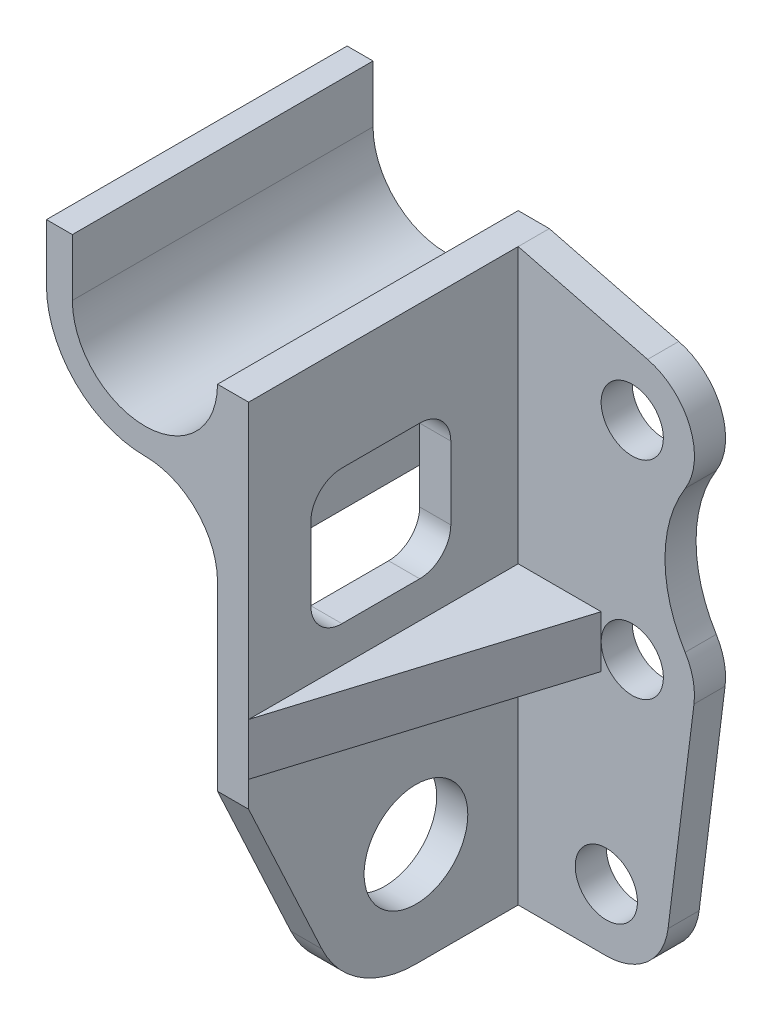
ISO-10303-21;
HEADER;
FILE_DESCRIPTION(('STEP AP214'),'2;1');
FILE_NAME('part.step','',(''),(''),'','','');
FILE_SCHEMA(('AUTOMOTIVE_DESIGN { 1 0 10303 214 1 1 1 1 }'));
ENDSEC;
DATA;
#1=APPLICATION_CONTEXT('core data for automotive mechanical design processes');
#2=APPLICATION_PROTOCOL_DEFINITION('international standard','automotive_design',2000,#1);
#3=PRODUCT_CONTEXT('',#1,'mechanical');
#4=PRODUCT('Part','Part','',(#3));
#5=PRODUCT_RELATED_PRODUCT_CATEGORY('part','',(#4));
#6=PRODUCT_DEFINITION_FORMATION('','',#4);
#7=PRODUCT_DEFINITION_CONTEXT('part definition',#1,'design');
#8=PRODUCT_DEFINITION('design','',#6,#7);
#9=PRODUCT_DEFINITION_SHAPE('','',#8);
#10=(LENGTH_UNIT() NAMED_UNIT(*) SI_UNIT(.MILLI.,.METRE.));
#11=(NAMED_UNIT(*) PLANE_ANGLE_UNIT() SI_UNIT($,.RADIAN.));
#12=(NAMED_UNIT(*) SI_UNIT($,.STERADIAN.) SOLID_ANGLE_UNIT());
#13=UNCERTAINTY_MEASURE_WITH_UNIT(LENGTH_MEASURE(1.E-05),#10,'distance_accuracy_value','');
#14=(GEOMETRIC_REPRESENTATION_CONTEXT(3) GLOBAL_UNCERTAINTY_ASSIGNED_CONTEXT((#13)) GLOBAL_UNIT_ASSIGNED_CONTEXT((#10,
#11,#12)) REPRESENTATION_CONTEXT('',''));
#15=CARTESIAN_POINT('',(0.,0.,0.));
#16=DIRECTION('',(0.,0.,1.));
#17=DIRECTION('',(1.,0.,0.));
#18=AXIS2_PLACEMENT_3D('',#15,#16,#17);
#19=CARTESIAN_POINT('',(6.,-90.,25.7215081756419));
#20=DIRECTION('',(1.,0.,0.));
#21=DIRECTION('',(0.,0.,-1.));
#22=AXIS2_PLACEMENT_3D('',#19,#20,#21);
#23=PLANE('',#22);
#24=CARTESIAN_POINT('',(6.,-90.,25.7215081756419));
#25=DIRECTION('',(1.,0.,0.));
#26=DIRECTION('',(0.,0.,-1.));
#27=AXIS2_PLACEMENT_3D('',#24,#25,#26);
#28=CIRCLE('',#27,10.);
#29=CARTESIAN_POINT('',(6.,-90.,15.7215081756419));
#30=VERTEX_POINT('',#29);
#31=EDGE_CURVE('E389',#30,#30,#28,.T.);
#32=ORIENTED_EDGE('',*,*,#31,.F.);
#33=EDGE_LOOP('',(#32));
#34=FACE_BOUND('',#33,.T.);
#35=DIRECTION('',(0.,1.,0.));
#36=VECTOR('',#35,1.);
#37=CARTESIAN_POINT('',(6.,-18.,6.));
#38=LINE('',#37,#36);
#39=CARTESIAN_POINT('',(6.,-110.,6.));
#40=VERTEX_POINT('',#39);
#41=CARTESIAN_POINT('',(6.,-63.,6.));
#42=VERTEX_POINT('',#41);
#43=EDGE_CURVE('E424',#40,#42,#38,.T.);
#44=ORIENTED_EDGE('',*,*,#43,.T.);
#45=DIRECTION('',(0.,0.,1.));
#46=VECTOR('',#45,1.);
#47=CARTESIAN_POINT('',(6.,-63.,25.7215081756419));
#48=LINE('',#47,#46);
#49=CARTESIAN_POINT('',(6.,-63.,58.));
#50=VERTEX_POINT('',#49);
#51=EDGE_CURVE('E309',#42,#50,#48,.T.);
#52=ORIENTED_EDGE('',*,*,#51,.T.);
#53=DIRECTION('',(0.,-1.,0.));
#54=VECTOR('',#53,1.);
#55=CARTESIAN_POINT('',(6.,0.,58.));
#56=LINE('',#55,#54);
#57=CARTESIAN_POINT('',(6.,-68.,58.));
#58=VERTEX_POINT('',#57);
#59=EDGE_CURVE('E391',#50,#58,#56,.T.);
#60=ORIENTED_EDGE('',*,*,#59,.T.);
#61=DIRECTION('',(0.,-0.906852855395933,-0.4214473853997));
#62=VECTOR('',#61,1.);
#63=CARTESIAN_POINT('',(6.,-68.,58.));
#64=LINE('',#63,#62);
#65=CARTESIAN_POINT('',(6.,-98.428947707994,43.8585652835606));
#66=VERTEX_POINT('',#65);
#67=EDGE_CURVE('E396',#58,#66,#64,.T.);
#68=ORIENTED_EDGE('',*,*,#67,.T.);
#69=CARTESIAN_POINT('',(6.,-90.,25.7215081756419));
#70=DIRECTION('',(1.,0.,0.));
#71=DIRECTION('',(0.,0.,-1.));
#72=AXIS2_PLACEMENT_3D('',#69,#70,#71);
#73=CIRCLE('',#72,20.);
#74=CARTESIAN_POINT('',(6.,-110.,25.7215081756419));
#75=VERTEX_POINT('',#74);
#76=EDGE_CURVE('E401',#66,#75,#73,.T.);
#77=ORIENTED_EDGE('',*,*,#76,.T.);
#78=DIRECTION('',(0.,0.,-1.));
#79=VECTOR('',#78,1.);
#80=CARTESIAN_POINT('',(6.,-110.,5.7215081756419));
#81=LINE('',#80,#79);
#82=EDGE_CURVE('E403',#75,#40,#81,.T.);
#83=ORIENTED_EDGE('',*,*,#82,.T.);
#84=EDGE_LOOP('',(#44,#52,#60,#68,#77,#83));
#85=FACE_BOUND('',#84,.T.);
#86=ADVANCED_FACE('F44',(#34,#85),#23,.T.);
#87=CARTESIAN_POINT('',(28.,-18.,6.));
#88=DIRECTION('',(0.,0.,1.));
#89=DIRECTION('',(1.,0.,0.));
#90=AXIS2_PLACEMENT_3D('',#87,#88,#89);
#91=PLANE('',#90);
#92=DIRECTION('',(-1.,0.,0.));
#93=VECTOR('',#92,1.);
#94=CARTESIAN_POINT('',(28.,-53.,6.));
#95=LINE('',#94,#93);
#96=CARTESIAN_POINT('',(22.,-53.,6.));
#97=VERTEX_POINT('',#96);
#98=CARTESIAN_POINT('',(6.,-53.,6.));
#99=VERTEX_POINT('',#98);
#100=EDGE_CURVE('E319',#97,#99,#95,.T.);
#101=ORIENTED_EDGE('',*,*,#100,.F.);
#102=DIRECTION('',(0.,1.,0.));
#103=VECTOR('',#102,1.);
#104=CARTESIAN_POINT('',(22.,-18.,6.));
#105=LINE('',#104,#103);
#106=CARTESIAN_POINT('',(22.,-58.,6.));
#107=VERTEX_POINT('',#106);
#108=EDGE_CURVE('E323',#107,#97,#105,.T.);
#109=ORIENTED_EDGE('',*,*,#108,.F.);
#110=CARTESIAN_POINT('',(28.,-58.,6.));
#111=DIRECTION('',(0.,0.,1.));
#112=DIRECTION('',(1.,0.,0.));
#113=AXIS2_PLACEMENT_3D('',#110,#111,#112);
#114=CIRCLE('',#113,6.);
#115=EDGE_CURVE('E439',#107,#107,#114,.T.);
#116=ORIENTED_EDGE('',*,*,#115,.F.);
#117=CARTESIAN_POINT('',(22.,-63.,6.));
#118=VERTEX_POINT('',#117);
#119=EDGE_CURVE('E326',#118,#107,#105,.T.);
#120=ORIENTED_EDGE('',*,*,#119,.F.);
#121=DIRECTION('',(-1.,0.,0.));
#122=VECTOR('',#121,1.);
#123=CARTESIAN_POINT('',(28.,-63.,6.));
#124=LINE('',#123,#122);
#125=EDGE_CURVE('E312',#118,#42,#124,.T.);
#126=ORIENTED_EDGE('',*,*,#125,.T.);
#127=ORIENTED_EDGE('',*,*,#43,.F.);
#128=DIRECTION('',(1.,0.,0.));
#129=VECTOR('',#128,1.);
#130=CARTESIAN_POINT('',(23.,-110.,6.));
#131=LINE('',#130,#129);
#132=CARTESIAN_POINT('',(23.,-110.,6.));
#133=VERTEX_POINT('',#132);
#134=EDGE_CURVE('E448',#40,#133,#131,.T.);
#135=ORIENTED_EDGE('',*,*,#134,.T.);
#136=CARTESIAN_POINT('',(23.,-98.,6.));
#137=DIRECTION('',(0.,0.,1.));
#138=DIRECTION('',(1.,0.,0.));
#139=AXIS2_PLACEMENT_3D('',#136,#137,#138);
#140=CIRCLE('',#139,12.);
#141=CARTESIAN_POINT('',(34.907334520564,-99.4884168150705,6.));
#142=VERTEX_POINT('',#141);
#143=EDGE_CURVE('E447',#133,#142,#140,.T.);
#144=ORIENTED_EDGE('',*,*,#143,.T.);
#145=DIRECTION('',(0.124034734589208,0.992277876713668,0.));
#146=VECTOR('',#145,1.);
#147=CARTESIAN_POINT('',(34.907334520564,-99.4884168150705,6.));
#148=LINE('',#147,#146);
#149=CARTESIAN_POINT('',(39.907334520564,-59.4884168150705,6.));
#150=VERTEX_POINT('',#149);
#151=EDGE_CURVE('E452',#142,#150,#148,.T.);
#152=ORIENTED_EDGE('',*,*,#151,.T.);
#153=CARTESIAN_POINT('',(28.,-58.,6.));
#154=DIRECTION('',(0.,0.,1.));
#155=DIRECTION('',(1.,0.,0.));
#156=AXIS2_PLACEMENT_3D('',#153,#154,#155);
#157=CIRCLE('',#156,12.);
#158=CARTESIAN_POINT('',(38.2034701608864,-51.6842105263158,6.));
#159=VERTEX_POINT('',#158);
#160=EDGE_CURVE('E453',#150,#159,#157,.T.);
#161=ORIENTED_EDGE('',*,*,#160,.T.);
#162=CARTESIAN_POINT('',(60.310988842807,-38.,6.));
#163=DIRECTION('',(0.,0.,-1.));
#164=DIRECTION('',(-1.,0.,0.));
#165=AXIS2_PLACEMENT_3D('',#162,#163,#164);
#166=CIRCLE('',#165,26.);
#167=CARTESIAN_POINT('',(38.2034701608864,-24.3157894736842,6.));
#168=VERTEX_POINT('',#167);
#169=EDGE_CURVE('E451',#159,#168,#166,.T.);
#170=ORIENTED_EDGE('',*,*,#169,.T.);
#171=CARTESIAN_POINT('',(28.,-18.,6.));
#172=DIRECTION('',(0.,0.,1.));
#173=DIRECTION('',(1.,0.,0.));
#174=AXIS2_PLACEMENT_3D('',#171,#172,#173);
#175=CIRCLE('',#174,12.);
#176=CARTESIAN_POINT('',(30.9677359529026,-6.37276716867469,6.));
#177=VERTEX_POINT('',#176);
#178=EDGE_CURVE('E460',#168,#177,#175,.T.);
#179=ORIENTED_EDGE('',*,*,#178,.T.);
#180=DIRECTION('',(-0.968936069277111,0.247311329408546,0.));
#181=VECTOR('',#180,1.);
#182=CARTESIAN_POINT('',(6.,0.,6.));
#183=LINE('',#182,#181);
#184=CARTESIAN_POINT('',(6.,0.,6.));
#185=VERTEX_POINT('',#184);
#186=EDGE_CURVE('E459',#177,#185,#183,.T.);
#187=ORIENTED_EDGE('',*,*,#186,.T.);
#188=EDGE_CURVE('E421',#99,#185,#38,.T.);
#189=ORIENTED_EDGE('',*,*,#188,.F.);
#190=EDGE_LOOP('',(#101,#109,#116,#120,#126,#127,#135,#144,#152,#161,#170,#179,#187,#189));
#191=FACE_BOUND('',#190,.T.);
#192=CARTESIAN_POINT('',(23.,-98.,6.));
#193=DIRECTION('',(0.,0.,1.));
#194=DIRECTION('',(1.,0.,0.));
#195=AXIS2_PLACEMENT_3D('',#192,#193,#194);
#196=CIRCLE('',#195,6.);
#197=CARTESIAN_POINT('',(29.,-98.,6.));
#198=VERTEX_POINT('',#197);
#199=EDGE_CURVE('E432',#198,#198,#196,.T.);
#200=ORIENTED_EDGE('',*,*,#199,.F.);
#201=EDGE_LOOP('',(#200));
#202=FACE_BOUND('',#201,.T.);
#203=CARTESIAN_POINT('',(28.,-18.,6.));
#204=DIRECTION('',(0.,0.,1.));
#205=DIRECTION('',(1.,0.,0.));
#206=AXIS2_PLACEMENT_3D('',#203,#204,#205);
#207=CIRCLE('',#206,6.);
#208=CARTESIAN_POINT('',(34.,-18.,6.));
#209=VERTEX_POINT('',#208);
#210=EDGE_CURVE('E428',#209,#209,#207,.T.);
#211=ORIENTED_EDGE('',*,*,#210,.F.);
#212=EDGE_LOOP('',(#211));
#213=FACE_BOUND('',#212,.T.);
#214=ADVANCED_FACE('F525',(#191,#202,#213),#91,.T.);
#215=CARTESIAN_POINT('',(28.,-18.,0.));
#216=DIRECTION('',(0.,0.,1.));
#217=DIRECTION('',(1.,0.,0.));
#218=AXIS2_PLACEMENT_3D('',#215,#216,#217);
#219=PLANE('',#218);
#220=CARTESIAN_POINT('',(28.,-58.,0.));
#221=DIRECTION('',(0.,0.,1.));
#222=DIRECTION('',(1.,0.,0.));
#223=AXIS2_PLACEMENT_3D('',#220,#221,#222);
#224=CIRCLE('',#223,6.);
#225=CARTESIAN_POINT('',(34.,-58.,0.));
#226=VERTEX_POINT('',#225);
#227=EDGE_CURVE('E440',#226,#226,#224,.T.);
#228=ORIENTED_EDGE('',*,*,#227,.T.);
#229=EDGE_LOOP('',(#228));
#230=FACE_BOUND('',#229,.T.);
#231=DIRECTION('',(1.,0.,0.));
#232=VECTOR('',#231,1.);
#233=CARTESIAN_POINT('',(23.,-110.,0.));
#234=LINE('',#233,#232);
#235=CARTESIAN_POINT('',(0.,-110.,0.));
#236=VERTEX_POINT('',#235);
#237=CARTESIAN_POINT('',(23.,-110.,0.));
#238=VERTEX_POINT('',#237);
#239=EDGE_CURVE('E465',#236,#238,#234,.T.);
#240=ORIENTED_EDGE('',*,*,#239,.F.);
#241=DIRECTION('',(0.,-1.,0.));
#242=VECTOR('',#241,1.);
#243=CARTESIAN_POINT('',(0.,-110.,0.));
#244=LINE('',#243,#242);
#245=CARTESIAN_POINT('',(0.,-33.,0.));
#246=VERTEX_POINT('',#245);
#247=EDGE_CURVE('E444',#246,#236,#244,.T.);
#248=ORIENTED_EDGE('',*,*,#247,.F.);
#249=CARTESIAN_POINT('',(-14.,-33.,0.));
#250=DIRECTION('',(0.,0.,1.));
#251=DIRECTION('',(1.,0.,0.));
#252=AXIS2_PLACEMENT_3D('',#249,#250,#251);
#253=CIRCLE('',#252,14.);
#254=CARTESIAN_POINT('',(-14.,-19.,0.));
#255=VERTEX_POINT('',#254);
#256=EDGE_CURVE('E537',#246,#255,#253,.T.);
#257=ORIENTED_EDGE('',*,*,#256,.T.);
#258=CARTESIAN_POINT('',(-14.,0.,0.));
#259=DIRECTION('',(0.,0.,1.));
#260=DIRECTION('',(1.,0.,0.));
#261=AXIS2_PLACEMENT_3D('',#258,#259,#260);
#262=CIRCLE('',#261,19.);
#263=CARTESIAN_POINT('',(-33.,0.,0.));
#264=VERTEX_POINT('',#263);
#265=EDGE_CURVE('E546',#255,#264,#262,.F.);
#266=ORIENTED_EDGE('',*,*,#265,.T.);
#267=DIRECTION('',(0.,1.,0.));
#268=VECTOR('',#267,1.);
#269=CARTESIAN_POINT('',(-33.,0.,0.));
#270=LINE('',#269,#268);
#271=CARTESIAN_POINT('',(-33.,11.,0.));
#272=VERTEX_POINT('',#271);
#273=EDGE_CURVE('E550',#264,#272,#270,.T.);
#274=ORIENTED_EDGE('',*,*,#273,.T.);
#275=DIRECTION('',(1.,0.,0.));
#276=VECTOR('',#275,1.);
#277=CARTESIAN_POINT('',(-33.,11.,0.));
#278=LINE('',#277,#276);
#279=CARTESIAN_POINT('',(-28.,11.,0.));
#280=VERTEX_POINT('',#279);
#281=EDGE_CURVE('E292',#272,#280,#278,.T.);
#282=ORIENTED_EDGE('',*,*,#281,.T.);
#283=DIRECTION('',(0.,-1.,0.));
#284=VECTOR('',#283,1.);
#285=CARTESIAN_POINT('',(-28.,11.,0.));
#286=LINE('',#285,#284);
#287=CARTESIAN_POINT('',(-28.,0.,0.));
#288=VERTEX_POINT('',#287);
#289=EDGE_CURVE('E302',#280,#288,#286,.T.);
#290=ORIENTED_EDGE('',*,*,#289,.T.);
#291=CARTESIAN_POINT('',(-14.,0.,0.));
#292=DIRECTION('',(0.,0.,1.));
#293=DIRECTION('',(1.,0.,0.));
#294=AXIS2_PLACEMENT_3D('',#291,#292,#293);
#295=CIRCLE('',#294,14.);
#296=CARTESIAN_POINT('',(0.,0.,0.));
#297=VERTEX_POINT('',#296);
#298=EDGE_CURVE('E260',#288,#297,#295,.T.);
#299=ORIENTED_EDGE('',*,*,#298,.T.);
#300=DIRECTION('',(-1.,0.,0.));
#301=VECTOR('',#300,1.);
#302=CARTESIAN_POINT('',(0.,0.,0.));
#303=LINE('',#302,#301);
#304=CARTESIAN_POINT('',(6.,0.,0.));
#305=VERTEX_POINT('',#304);
#306=EDGE_CURVE('E450',#305,#297,#303,.T.);
#307=ORIENTED_EDGE('',*,*,#306,.F.);
#308=DIRECTION('',(-0.968936069277111,0.247311329408546,0.));
#309=VECTOR('',#308,1.);
#310=CARTESIAN_POINT('',(6.,0.,0.));
#311=LINE('',#310,#309);
#312=CARTESIAN_POINT('',(30.9677359529026,-6.37276716867469,0.));
#313=VERTEX_POINT('',#312);
#314=EDGE_CURVE('E478',#313,#305,#311,.T.);
#315=ORIENTED_EDGE('',*,*,#314,.F.);
#316=CARTESIAN_POINT('',(28.,-18.,0.));
#317=DIRECTION('',(0.,0.,1.));
#318=DIRECTION('',(1.,0.,0.));
#319=AXIS2_PLACEMENT_3D('',#316,#317,#318);
#320=CIRCLE('',#319,12.);
#321=CARTESIAN_POINT('',(38.2034701608864,-24.3157894736842,0.));
#322=VERTEX_POINT('',#321);
#323=EDGE_CURVE('E475',#322,#313,#320,.T.);
#324=ORIENTED_EDGE('',*,*,#323,.F.);
#325=CARTESIAN_POINT('',(60.310988842807,-38.,0.));
#326=DIRECTION('',(0.,0.,-1.));
#327=DIRECTION('',(-1.,0.,0.));
#328=AXIS2_PLACEMENT_3D('',#325,#326,#327);
#329=CIRCLE('',#328,26.);
#330=CARTESIAN_POINT('',(38.2034701608864,-51.6842105263158,0.));
#331=VERTEX_POINT('',#330);
#332=EDGE_CURVE('E472',#331,#322,#329,.T.);
#333=ORIENTED_EDGE('',*,*,#332,.F.);
#334=CARTESIAN_POINT('',(28.,-58.,0.));
#335=DIRECTION('',(0.,0.,1.));
#336=DIRECTION('',(1.,0.,0.));
#337=AXIS2_PLACEMENT_3D('',#334,#335,#336);
#338=CIRCLE('',#337,12.);
#339=CARTESIAN_POINT('',(39.907334520564,-59.4884168150705,0.));
#340=VERTEX_POINT('',#339);
#341=EDGE_CURVE('E466',#340,#331,#338,.T.);
#342=ORIENTED_EDGE('',*,*,#341,.F.);
#343=DIRECTION('',(0.124034734589208,0.992277876713668,0.));
#344=VECTOR('',#343,1.);
#345=CARTESIAN_POINT('',(34.907334520564,-99.4884168150705,0.));
#346=LINE('',#345,#344);
#347=CARTESIAN_POINT('',(34.907334520564,-99.4884168150705,0.));
#348=VERTEX_POINT('',#347);
#349=EDGE_CURVE('E468',#348,#340,#346,.T.);
#350=ORIENTED_EDGE('',*,*,#349,.F.);
#351=CARTESIAN_POINT('',(23.,-98.,0.));
#352=DIRECTION('',(0.,0.,1.));
#353=DIRECTION('',(1.,0.,0.));
#354=AXIS2_PLACEMENT_3D('',#351,#352,#353);
#355=CIRCLE('',#354,12.);
#356=EDGE_CURVE('E467',#238,#348,#355,.T.);
#357=ORIENTED_EDGE('',*,*,#356,.F.);
#358=EDGE_LOOP('',(#240,#248,#257,#266,#274,#282,#290,#299,#307,#315,#324,#333,#342,#350,#357));
#359=FACE_BOUND('',#358,.T.);
#360=CARTESIAN_POINT('',(23.,-98.,0.));
#361=DIRECTION('',(0.,0.,1.));
#362=DIRECTION('',(1.,0.,0.));
#363=AXIS2_PLACEMENT_3D('',#360,#361,#362);
#364=CIRCLE('',#363,6.);
#365=CARTESIAN_POINT('',(29.,-98.,0.));
#366=VERTEX_POINT('',#365);
#367=EDGE_CURVE('E431',#366,#366,#364,.T.);
#368=ORIENTED_EDGE('',*,*,#367,.T.);
#369=EDGE_LOOP('',(#368));
#370=FACE_BOUND('',#369,.T.);
#371=CARTESIAN_POINT('',(28.,-18.,0.));
#372=DIRECTION('',(0.,0.,1.));
#373=DIRECTION('',(1.,0.,0.));
#374=AXIS2_PLACEMENT_3D('',#371,#372,#373);
#375=CIRCLE('',#374,6.);
#376=CARTESIAN_POINT('',(34.,-18.,0.));
#377=VERTEX_POINT('',#376);
#378=EDGE_CURVE('E430',#377,#377,#375,.T.);
#379=ORIENTED_EDGE('',*,*,#378,.T.);
#380=EDGE_LOOP('',(#379));
#381=FACE_BOUND('',#380,.T.);
#382=ADVANCED_FACE('F508',(#230,#359,#370,#381),#219,.F.);
#383=CARTESIAN_POINT('',(0.,-110.,6.));
#384=DIRECTION('',(1.,0.,0.));
#385=DIRECTION('',(0.,0.,-1.));
#386=AXIS2_PLACEMENT_3D('',#383,#384,#385);
#387=PLANE('',#386);
#388=DIRECTION('',(0.,-1.,0.));
#389=VECTOR('',#388,1.);
#390=CARTESIAN_POINT('',(0.,0.,58.));
#391=LINE('',#390,#389);
#392=CARTESIAN_POINT('',(0.,-33.,58.));
#393=VERTEX_POINT('',#392);
#394=CARTESIAN_POINT('',(0.,-68.,58.));
#395=VERTEX_POINT('',#394);
#396=EDGE_CURVE('E70',#393,#395,#391,.T.);
#397=ORIENTED_EDGE('',*,*,#396,.F.);
#398=DIRECTION('',(0.,0.,1.));
#399=VECTOR('',#398,1.);
#400=CARTESIAN_POINT('',(0.,-33.,-55.));
#401=LINE('',#400,#399);
#402=CARTESIAN_POINT('',(0.,-33.,46.));
#403=VERTEX_POINT('',#402);
#404=EDGE_CURVE('E291',#403,#393,#401,.T.);
#405=ORIENTED_EDGE('',*,*,#404,.F.);
#406=DIRECTION('',(0.,-1.,0.));
#407=VECTOR('',#406,1.);
#408=CARTESIAN_POINT('',(0.,-40.,46.));
#409=LINE('',#408,#407);
#410=CARTESIAN_POINT('',(0.,-40.,46.));
#411=VERTEX_POINT('',#410);
#412=EDGE_CURVE('E356',#403,#411,#409,.T.);
#413=ORIENTED_EDGE('',*,*,#412,.T.);
#414=CARTESIAN_POINT('',(0.,-40.,40.));
#415=DIRECTION('',(1.,0.,0.));
#416=DIRECTION('',(0.,0.,1.));
#417=AXIS2_PLACEMENT_3D('',#414,#415,#416);
#418=CIRCLE('',#417,6.);
#419=CARTESIAN_POINT('',(0.,-46.,40.));
#420=VERTEX_POINT('',#419);
#421=EDGE_CURVE('E365',#411,#420,#418,.T.);
#422=ORIENTED_EDGE('',*,*,#421,.T.);
#423=DIRECTION('',(0.,0.,-1.));
#424=VECTOR('',#423,1.);
#425=CARTESIAN_POINT('',(0.,-46.,40.));
#426=LINE('',#425,#424);
#427=CARTESIAN_POINT('',(0.,-46.,25.));
#428=VERTEX_POINT('',#427);
#429=EDGE_CURVE('E329',#420,#428,#426,.T.);
#430=ORIENTED_EDGE('',*,*,#429,.T.);
#431=CARTESIAN_POINT('',(0.,-40.,25.));
#432=DIRECTION('',(1.,0.,0.));
#433=DIRECTION('',(0.,0.,-1.));
#434=AXIS2_PLACEMENT_3D('',#431,#432,#433);
#435=CIRCLE('',#434,6.);
#436=CARTESIAN_POINT('',(0.,-40.,19.));
#437=VERTEX_POINT('',#436);
#438=EDGE_CURVE('E347',#428,#437,#435,.T.);
#439=ORIENTED_EDGE('',*,*,#438,.T.);
#440=DIRECTION('',(0.,1.,0.));
#441=VECTOR('',#440,1.);
#442=CARTESIAN_POINT('',(0.,-40.,19.));
#443=LINE('',#442,#441);
#444=CARTESIAN_POINT('',(0.,-33.,19.));
#445=VERTEX_POINT('',#444);
#446=EDGE_CURVE('E349',#437,#445,#443,.T.);
#447=ORIENTED_EDGE('',*,*,#446,.T.);
#448=EDGE_CURVE('E58',#246,#445,#401,.T.);
#449=ORIENTED_EDGE('',*,*,#448,.F.);
#450=ORIENTED_EDGE('',*,*,#247,.T.);
#451=DIRECTION('',(0.,0.,-1.));
#452=VECTOR('',#451,1.);
#453=CARTESIAN_POINT('',(0.,-110.,6.));
#454=LINE('',#453,#452);
#455=CARTESIAN_POINT('',(0.,-110.,25.7215081756419));
#456=VERTEX_POINT('',#455);
#457=EDGE_CURVE('E11',#456,#236,#454,.T.);
#458=ORIENTED_EDGE('',*,*,#457,.F.);
#459=CARTESIAN_POINT('',(0.,-90.,25.7215081756419));
#460=DIRECTION('',(1.,0.,0.));
#461=DIRECTION('',(0.,0.,-1.));
#462=AXIS2_PLACEMENT_3D('',#459,#460,#461);
#463=CIRCLE('',#462,20.);
#464=CARTESIAN_POINT('',(0.,-98.428947707994,43.8585652835606));
#465=VERTEX_POINT('',#464);
#466=EDGE_CURVE('E397',#465,#456,#463,.T.);
#467=ORIENTED_EDGE('',*,*,#466,.F.);
#468=DIRECTION('',(0.,-0.906852855395933,-0.4214473853997));
#469=VECTOR('',#468,1.);
#470=CARTESIAN_POINT('',(0.,-68.,58.));
#471=LINE('',#470,#469);
#472=EDGE_CURVE('E406',#395,#465,#471,.T.);
#473=ORIENTED_EDGE('',*,*,#472,.F.);
#474=EDGE_LOOP('',(#397,#405,#413,#422,#430,#439,#447,#449,#450,#458,#467,#473));
#475=FACE_BOUND('',#474,.T.);
#476=CARTESIAN_POINT('',(0.,-90.,25.7215081756419));
#477=DIRECTION('',(1.,0.,0.));
#478=DIRECTION('',(0.,0.,-1.));
#479=AXIS2_PLACEMENT_3D('',#476,#477,#478);
#480=CIRCLE('',#479,10.);
#481=CARTESIAN_POINT('',(0.,-90.,15.7215081756419));
#482=VERTEX_POINT('',#481);
#483=EDGE_CURVE('E390',#482,#482,#480,.T.);
#484=ORIENTED_EDGE('',*,*,#483,.T.);
#485=EDGE_LOOP('',(#484));
#486=FACE_BOUND('',#485,.T.);
#487=ADVANCED_FACE('F50',(#475,#486),#387,.F.);
#488=CARTESIAN_POINT('',(23.,-110.,6.));
#489=DIRECTION('',(0.,1.,0.));
#490=DIRECTION('',(0.,0.,1.));
#491=AXIS2_PLACEMENT_3D('',#488,#489,#490);
#492=PLANE('',#491);
#493=ORIENTED_EDGE('',*,*,#134,.F.);
#494=ORIENTED_EDGE('',*,*,#82,.F.);
#495=DIRECTION('',(-1.,0.,0.));
#496=VECTOR('',#495,1.);
#497=CARTESIAN_POINT('',(6.,-110.,25.7215081756419));
#498=LINE('',#497,#496);
#499=EDGE_CURVE('E407',#75,#456,#498,.T.);
#500=ORIENTED_EDGE('',*,*,#499,.T.);
#501=ORIENTED_EDGE('',*,*,#457,.T.);
#502=ORIENTED_EDGE('',*,*,#239,.T.);
#503=DIRECTION('',(0.,0.,-1.));
#504=VECTOR('',#503,1.);
#505=CARTESIAN_POINT('',(23.,-110.,6.));
#506=LINE('',#505,#504);
#507=EDGE_CURVE('E52',#133,#238,#506,.T.);
#508=ORIENTED_EDGE('',*,*,#507,.F.);
#509=EDGE_LOOP('',(#493,#494,#500,#501,#502,#508));
#510=FACE_BOUND('',#509,.T.);
#511=ADVANCED_FACE('F527',(#510),#492,.F.);
#512=CARTESIAN_POINT('',(23.,-98.,6.));
#513=DIRECTION('',(0.,0.,-1.));
#514=DIRECTION('',(-1.,0.,0.));
#515=AXIS2_PLACEMENT_3D('',#512,#513,#514);
#516=CYLINDRICAL_SURFACE('',#515,12.);
#517=ORIENTED_EDGE('',*,*,#356,.T.);
#518=DIRECTION('',(0.,0.,-1.));
#519=VECTOR('',#518,1.);
#520=CARTESIAN_POINT('',(34.907334520564,-99.4884168150705,6.));
#521=LINE('',#520,#519);
#522=EDGE_CURVE('E494',#142,#348,#521,.T.);
#523=ORIENTED_EDGE('',*,*,#522,.F.);
#524=ORIENTED_EDGE('',*,*,#143,.F.);
#525=ORIENTED_EDGE('',*,*,#507,.T.);
#526=EDGE_LOOP('',(#517,#523,#524,#525));
#527=FACE_BOUND('',#526,.T.);
#528=ADVANCED_FACE('F504',(#527),#516,.T.);
#529=CARTESIAN_POINT('',(34.907334520564,-99.4884168150705,6.));
#530=DIRECTION('',(-0.992277876713668,0.124034734589208,0.));
#531=DIRECTION('',(-0.124034734589208,-0.992277876713668,0.));
#532=AXIS2_PLACEMENT_3D('',#529,#530,#531);
#533=PLANE('',#532);
#534=ORIENTED_EDGE('',*,*,#349,.T.);
#535=DIRECTION('',(0.,0.,-1.));
#536=VECTOR('',#535,1.);
#537=CARTESIAN_POINT('',(39.907334520564,-59.4884168150705,6.));
#538=LINE('',#537,#536);
#539=EDGE_CURVE('E495',#150,#340,#538,.T.);
#540=ORIENTED_EDGE('',*,*,#539,.F.);
#541=ORIENTED_EDGE('',*,*,#151,.F.);
#542=ORIENTED_EDGE('',*,*,#522,.T.);
#543=EDGE_LOOP('',(#534,#540,#541,#542));
#544=FACE_BOUND('',#543,.T.);
#545=ADVANCED_FACE('F514',(#544),#533,.F.);
#546=CARTESIAN_POINT('',(28.,-58.,6.));
#547=DIRECTION('',(0.,0.,-1.));
#548=DIRECTION('',(-1.,0.,0.));
#549=AXIS2_PLACEMENT_3D('',#546,#547,#548);
#550=CYLINDRICAL_SURFACE('',#549,12.);
#551=ORIENTED_EDGE('',*,*,#341,.T.);
#552=DIRECTION('',(0.,0.,-1.));
#553=VECTOR('',#552,1.);
#554=CARTESIAN_POINT('',(38.2034701608864,-51.6842105263158,6.));
#555=LINE('',#554,#553);
#556=EDGE_CURVE('E487',#159,#331,#555,.T.);
#557=ORIENTED_EDGE('',*,*,#556,.F.);
#558=ORIENTED_EDGE('',*,*,#160,.F.);
#559=ORIENTED_EDGE('',*,*,#539,.T.);
#560=EDGE_LOOP('',(#551,#557,#558,#559));
#561=FACE_BOUND('',#560,.T.);
#562=ADVANCED_FACE('F517',(#561),#550,.T.);
#563=CARTESIAN_POINT('',(60.310988842807,-38.,6.));
#564=DIRECTION('',(0.,0.,-1.));
#565=DIRECTION('',(-1.,0.,0.));
#566=AXIS2_PLACEMENT_3D('',#563,#564,#565);
#567=CYLINDRICAL_SURFACE('',#566,26.);
#568=ORIENTED_EDGE('',*,*,#332,.T.);
#569=DIRECTION('',(0.,0.,-1.));
#570=VECTOR('',#569,1.);
#571=CARTESIAN_POINT('',(38.2034701608864,-24.3157894736842,6.));
#572=LINE('',#571,#570);
#573=EDGE_CURVE('E486',#168,#322,#572,.T.);
#574=ORIENTED_EDGE('',*,*,#573,.F.);
#575=ORIENTED_EDGE('',*,*,#169,.F.);
#576=ORIENTED_EDGE('',*,*,#556,.T.);
#577=EDGE_LOOP('',(#568,#574,#575,#576));
#578=FACE_BOUND('',#577,.T.);
#579=ADVANCED_FACE('F684',(#578),#567,.F.);
#580=CARTESIAN_POINT('',(28.,-18.,6.));
#581=DIRECTION('',(0.,0.,-1.));
#582=DIRECTION('',(-1.,0.,0.));
#583=AXIS2_PLACEMENT_3D('',#580,#581,#582);
#584=CYLINDRICAL_SURFACE('',#583,12.);
#585=ORIENTED_EDGE('',*,*,#323,.T.);
#586=DIRECTION('',(0.,0.,-1.));
#587=VECTOR('',#586,1.);
#588=CARTESIAN_POINT('',(30.9677359529026,-6.37276716867469,6.));
#589=LINE('',#588,#587);
#590=EDGE_CURVE('E483',#177,#313,#589,.T.);
#591=ORIENTED_EDGE('',*,*,#590,.F.);
#592=ORIENTED_EDGE('',*,*,#178,.F.);
#593=ORIENTED_EDGE('',*,*,#573,.T.);
#594=EDGE_LOOP('',(#585,#591,#592,#593));
#595=FACE_BOUND('',#594,.T.);
#596=ADVANCED_FACE('F676',(#595),#584,.T.);
#597=CARTESIAN_POINT('',(6.,0.,6.));
#598=DIRECTION('',(-0.247311329408546,-0.968936069277111,0.));
#599=DIRECTION('',(0.968936069277111,-0.247311329408546,0.));
#600=AXIS2_PLACEMENT_3D('',#597,#598,#599);
#601=PLANE('',#600);
#602=ORIENTED_EDGE('',*,*,#314,.T.);
#603=DIRECTION('',(0.,0.,-1.));
#604=VECTOR('',#603,1.);
#605=CARTESIAN_POINT('',(6.,0.,6.));
#606=LINE('',#605,#604);
#607=EDGE_CURVE('E477',#185,#305,#606,.T.);
#608=ORIENTED_EDGE('',*,*,#607,.F.);
#609=ORIENTED_EDGE('',*,*,#186,.F.);
#610=ORIENTED_EDGE('',*,*,#590,.T.);
#611=EDGE_LOOP('',(#602,#608,#609,#610));
#612=FACE_BOUND('',#611,.T.);
#613=ADVANCED_FACE('F671',(#612),#601,.F.);
#614=CARTESIAN_POINT('',(0.,0.,6.));
#615=DIRECTION('',(0.,-1.,0.));
#616=DIRECTION('',(0.,0.,-1.));
#617=AXIS2_PLACEMENT_3D('',#614,#615,#616);
#618=PLANE('',#617);
#619=ORIENTED_EDGE('',*,*,#306,.T.);
#620=DIRECTION('',(0.,0.,-1.));
#621=VECTOR('',#620,1.);
#622=CARTESIAN_POINT('',(0.,0.,6.));
#623=LINE('',#622,#621);
#624=CARTESIAN_POINT('',(0.,0.,58.));
#625=VERTEX_POINT('',#624);
#626=EDGE_CURVE('E464',#625,#297,#623,.T.);
#627=ORIENTED_EDGE('',*,*,#626,.F.);
#628=DIRECTION('',(-1.,0.,0.));
#629=VECTOR('',#628,1.);
#630=CARTESIAN_POINT('',(6.,0.,58.));
#631=LINE('',#630,#629);
#632=CARTESIAN_POINT('',(6.,0.,58.));
#633=VERTEX_POINT('',#632);
#634=EDGE_CURVE('E277',#633,#625,#631,.T.);
#635=ORIENTED_EDGE('',*,*,#634,.F.);
#636=DIRECTION('',(0.,0.,1.));
#637=VECTOR('',#636,1.);
#638=CARTESIAN_POINT('',(6.,0.,0.));
#639=LINE('',#638,#637);
#640=EDGE_CURVE('E392',#185,#633,#639,.T.);
#641=ORIENTED_EDGE('',*,*,#640,.F.);
#642=ORIENTED_EDGE('',*,*,#607,.T.);
#643=EDGE_LOOP('',(#619,#627,#635,#641,#642));
#644=FACE_BOUND('',#643,.T.);
#645=ADVANCED_FACE('F675',(#644),#618,.F.);
#646=CARTESIAN_POINT('',(28.,-58.,6.));
#647=DIRECTION('',(0.,0.,-1.));
#648=DIRECTION('',(-1.,0.,0.));
#649=AXIS2_PLACEMENT_3D('',#646,#647,#648);
#650=CYLINDRICAL_SURFACE('',#649,6.);
#651=ORIENTED_EDGE('',*,*,#115,.T.);
#652=EDGE_LOOP('',(#651));
#653=FACE_BOUND('',#652,.T.);
#654=ORIENTED_EDGE('',*,*,#227,.F.);
#655=EDGE_LOOP('',(#654));
#656=FACE_BOUND('',#655,.T.);
#657=ADVANCED_FACE('F674',(#653,#656),#650,.F.);
#658=CARTESIAN_POINT('',(23.,-98.,6.));
#659=DIRECTION('',(0.,0.,-1.));
#660=DIRECTION('',(-1.,0.,0.));
#661=AXIS2_PLACEMENT_3D('',#658,#659,#660);
#662=CYLINDRICAL_SURFACE('',#661,6.);
#663=ORIENTED_EDGE('',*,*,#199,.T.);
#664=EDGE_LOOP('',(#663));
#665=FACE_BOUND('',#664,.T.);
#666=ORIENTED_EDGE('',*,*,#367,.F.);
#667=EDGE_LOOP('',(#666));
#668=FACE_BOUND('',#667,.T.);
#669=ADVANCED_FACE('F594',(#665,#668),#662,.F.);
#670=CARTESIAN_POINT('',(28.,-18.,6.));
#671=DIRECTION('',(0.,0.,-1.));
#672=DIRECTION('',(-1.,0.,0.));
#673=AXIS2_PLACEMENT_3D('',#670,#671,#672);
#674=CYLINDRICAL_SURFACE('',#673,6.);
#675=ORIENTED_EDGE('',*,*,#210,.T.);
#676=EDGE_LOOP('',(#675));
#677=FACE_BOUND('',#676,.T.);
#678=ORIENTED_EDGE('',*,*,#378,.F.);
#679=EDGE_LOOP('',(#678));
#680=FACE_BOUND('',#679,.T.);
#681=ADVANCED_FACE('F586',(#677,#680),#674,.F.);
#682=DIRECTION('',(0.,0.,1.));
#683=VECTOR('',#682,1.);
#684=CARTESIAN_POINT('',(6.,-53.,25.7215081756419));
#685=LINE('',#684,#683);
#686=CARTESIAN_POINT('',(6.,-53.,58.));
#687=VERTEX_POINT('',#686);
#688=EDGE_CURVE('E320',#99,#687,#685,.T.);
#689=ORIENTED_EDGE('',*,*,#688,.F.);
#690=ORIENTED_EDGE('',*,*,#188,.T.);
#691=ORIENTED_EDGE('',*,*,#640,.T.);
#692=EDGE_CURVE('E400',#633,#687,#56,.T.);
#693=ORIENTED_EDGE('',*,*,#692,.T.);
#694=EDGE_LOOP('',(#689,#690,#691,#693));
#695=FACE_BOUND('',#694,.T.);
#696=DIRECTION('',(0.,1.,0.));
#697=VECTOR('',#696,1.);
#698=CARTESIAN_POINT('',(6.,-40.,19.));
#699=LINE('',#698,#697);
#700=CARTESIAN_POINT('',(6.,-40.,19.));
#701=VERTEX_POINT('',#700);
#702=CARTESIAN_POINT('',(6.,-26.,19.));
#703=VERTEX_POINT('',#702);
#704=EDGE_CURVE('E328',#701,#703,#699,.T.);
#705=ORIENTED_EDGE('',*,*,#704,.F.);
#706=CARTESIAN_POINT('',(6.,-40.,25.));
#707=DIRECTION('',(1.,0.,0.));
#708=DIRECTION('',(0.,0.,-1.));
#709=AXIS2_PLACEMENT_3D('',#706,#707,#708);
#710=CIRCLE('',#709,6.);
#711=CARTESIAN_POINT('',(6.,-46.,25.));
#712=VERTEX_POINT('',#711);
#713=EDGE_CURVE('E330',#712,#701,#710,.T.);
#714=ORIENTED_EDGE('',*,*,#713,.F.);
#715=DIRECTION('',(0.,0.,-1.));
#716=VECTOR('',#715,1.);
#717=CARTESIAN_POINT('',(6.,-46.,40.));
#718=LINE('',#717,#716);
#719=CARTESIAN_POINT('',(6.,-46.,40.));
#720=VERTEX_POINT('',#719);
#721=EDGE_CURVE('E343',#720,#712,#718,.T.);
#722=ORIENTED_EDGE('',*,*,#721,.F.);
#723=CARTESIAN_POINT('',(6.,-40.,40.));
#724=DIRECTION('',(1.,0.,0.));
#725=DIRECTION('',(0.,0.,1.));
#726=AXIS2_PLACEMENT_3D('',#723,#724,#725);
#727=CIRCLE('',#726,6.);
#728=CARTESIAN_POINT('',(6.,-40.,46.));
#729=VERTEX_POINT('',#728);
#730=EDGE_CURVE('E336',#729,#720,#727,.T.);
#731=ORIENTED_EDGE('',*,*,#730,.F.);
#732=DIRECTION('',(0.,-1.,0.));
#733=VECTOR('',#732,1.);
#734=CARTESIAN_POINT('',(6.,-40.,46.));
#735=LINE('',#734,#733);
#736=CARTESIAN_POINT('',(6.,-26.,46.));
#737=VERTEX_POINT('',#736);
#738=EDGE_CURVE('E337',#737,#729,#735,.T.);
#739=ORIENTED_EDGE('',*,*,#738,.F.);
#740=CARTESIAN_POINT('',(6.,-26.,40.));
#741=DIRECTION('',(1.,0.,0.));
#742=DIRECTION('',(0.,0.,1.));
#743=AXIS2_PLACEMENT_3D('',#740,#741,#742);
#744=CIRCLE('',#743,6.);
#745=CARTESIAN_POINT('',(6.,-20.,40.));
#746=VERTEX_POINT('',#745);
#747=EDGE_CURVE('E338',#746,#737,#744,.T.);
#748=ORIENTED_EDGE('',*,*,#747,.F.);
#749=DIRECTION('',(0.,0.,1.));
#750=VECTOR('',#749,1.);
#751=CARTESIAN_POINT('',(6.,-20.,40.));
#752=LINE('',#751,#750);
#753=CARTESIAN_POINT('',(6.,-20.,25.));
#754=VERTEX_POINT('',#753);
#755=EDGE_CURVE('E331',#754,#746,#752,.T.);
#756=ORIENTED_EDGE('',*,*,#755,.F.);
#757=CARTESIAN_POINT('',(6.,-26.,25.));
#758=DIRECTION('',(1.,0.,0.));
#759=DIRECTION('',(0.,0.,1.));
#760=AXIS2_PLACEMENT_3D('',#757,#758,#759);
#761=CIRCLE('',#760,6.);
#762=EDGE_CURVE('E335',#703,#754,#761,.T.);
#763=ORIENTED_EDGE('',*,*,#762,.F.);
#764=EDGE_LOOP('',(#705,#714,#722,#731,#739,#748,#756,#763));
#765=FACE_BOUND('',#764,.T.);
#766=ADVANCED_FACE('F571',(#695,#765),#23,.T.);
#767=CARTESIAN_POINT('',(6.,0.,58.));
#768=DIRECTION('',(0.,0.,-1.));
#769=DIRECTION('',(0.,1.,0.));
#770=AXIS2_PLACEMENT_3D('',#767,#768,#769);
#771=PLANE('',#770);
#772=ORIENTED_EDGE('',*,*,#634,.T.);
#773=CARTESIAN_POINT('',(-14.,0.,58.));
#774=DIRECTION('',(0.,0.,-1.));
#775=DIRECTION('',(-1.,0.,0.));
#776=AXIS2_PLACEMENT_3D('',#773,#774,#775);
#777=CIRCLE('',#776,14.);
#778=CARTESIAN_POINT('',(-28.,0.,58.));
#779=VERTEX_POINT('',#778);
#780=EDGE_CURVE('E254',#625,#779,#777,.T.);
#781=ORIENTED_EDGE('',*,*,#780,.T.);
#782=DIRECTION('',(0.,1.,0.));
#783=VECTOR('',#782,1.);
#784=CARTESIAN_POINT('',(-28.,11.,58.));
#785=LINE('',#784,#783);
#786=CARTESIAN_POINT('',(-28.,11.,58.));
#787=VERTEX_POINT('',#786);
#788=EDGE_CURVE('E262',#779,#787,#785,.T.);
#789=ORIENTED_EDGE('',*,*,#788,.T.);
#790=DIRECTION('',(-1.,0.,0.));
#791=VECTOR('',#790,1.);
#792=CARTESIAN_POINT('',(-33.,11.,58.));
#793=LINE('',#792,#791);
#794=CARTESIAN_POINT('',(-33.,11.,58.));
#795=VERTEX_POINT('',#794);
#796=EDGE_CURVE('E269',#787,#795,#793,.T.);
#797=ORIENTED_EDGE('',*,*,#796,.T.);
#798=DIRECTION('',(0.,-1.,0.));
#799=VECTOR('',#798,1.);
#800=CARTESIAN_POINT('',(-33.,0.,58.));
#801=LINE('',#800,#799);
#802=CARTESIAN_POINT('',(-33.,0.,58.));
#803=VERTEX_POINT('',#802);
#804=EDGE_CURVE('E284',#795,#803,#801,.T.);
#805=ORIENTED_EDGE('',*,*,#804,.T.);
#806=CARTESIAN_POINT('',(-14.,0.,58.));
#807=DIRECTION('',(0.,0.,1.));
#808=DIRECTION('',(1.,0.,0.));
#809=AXIS2_PLACEMENT_3D('',#806,#807,#808);
#810=CIRCLE('',#809,19.);
#811=CARTESIAN_POINT('',(-14.,-19.,58.));
#812=VERTEX_POINT('',#811);
#813=EDGE_CURVE('E281',#803,#812,#810,.T.);
#814=ORIENTED_EDGE('',*,*,#813,.T.);
#815=CARTESIAN_POINT('',(-14.,-33.,58.));
#816=DIRECTION('',(0.,0.,-1.));
#817=DIRECTION('',(-1.,0.,0.));
#818=AXIS2_PLACEMENT_3D('',#815,#816,#817);
#819=CIRCLE('',#818,14.);
#820=EDGE_CURVE('E261',#812,#393,#819,.T.);
#821=ORIENTED_EDGE('',*,*,#820,.T.);
#822=ORIENTED_EDGE('',*,*,#396,.T.);
#823=DIRECTION('',(-1.,0.,0.));
#824=VECTOR('',#823,1.);
#825=CARTESIAN_POINT('',(6.,-68.,58.));
#826=LINE('',#825,#824);
#827=EDGE_CURVE('E420',#58,#395,#826,.T.);
#828=ORIENTED_EDGE('',*,*,#827,.F.);
#829=ORIENTED_EDGE('',*,*,#59,.F.);
#830=EDGE_CURVE('E402',#687,#50,#56,.T.);
#831=ORIENTED_EDGE('',*,*,#830,.F.);
#832=ORIENTED_EDGE('',*,*,#692,.F.);
#833=EDGE_LOOP('',(#772,#781,#789,#797,#805,#814,#821,#822,#828,#829,#831,#832));
#834=FACE_BOUND('',#833,.T.);
#835=ADVANCED_FACE('F272',(#834),#771,.F.);
#836=CARTESIAN_POINT('',(6.,-68.,58.));
#837=DIRECTION('',(0.,0.4214473853997,-0.906852855395933));
#838=DIRECTION('',(0.,0.906852855395933,0.4214473853997));
#839=AXIS2_PLACEMENT_3D('',#836,#837,#838);
#840=PLANE('',#839);
#841=ORIENTED_EDGE('',*,*,#472,.T.);
#842=DIRECTION('',(-1.,0.,0.));
#843=VECTOR('',#842,1.);
#844=CARTESIAN_POINT('',(6.,-98.428947707994,43.8585652835606));
#845=LINE('',#844,#843);
#846=EDGE_CURVE('E418',#66,#465,#845,.T.);
#847=ORIENTED_EDGE('',*,*,#846,.F.);
#848=ORIENTED_EDGE('',*,*,#67,.F.);
#849=ORIENTED_EDGE('',*,*,#827,.T.);
#850=EDGE_LOOP('',(#841,#847,#848,#849));
#851=FACE_BOUND('',#850,.T.);
#852=ADVANCED_FACE('F561',(#851),#840,.F.);
#853=CARTESIAN_POINT('',(6.,-90.,25.7215081756419));
#854=DIRECTION('',(-1.,0.,0.));
#855=DIRECTION('',(0.,0.,1.));
#856=AXIS2_PLACEMENT_3D('',#853,#854,#855);
#857=CYLINDRICAL_SURFACE('',#856,20.);
#858=ORIENTED_EDGE('',*,*,#466,.T.);
#859=ORIENTED_EDGE('',*,*,#499,.F.);
#860=ORIENTED_EDGE('',*,*,#76,.F.);
#861=ORIENTED_EDGE('',*,*,#846,.T.);
#862=EDGE_LOOP('',(#858,#859,#860,#861));
#863=FACE_BOUND('',#862,.T.);
#864=ADVANCED_FACE('F532',(#863),#857,.T.);
#865=CARTESIAN_POINT('',(6.,-90.,25.7215081756419));
#866=DIRECTION('',(-1.,0.,0.));
#867=DIRECTION('',(0.,0.,1.));
#868=AXIS2_PLACEMENT_3D('',#865,#866,#867);
#869=CYLINDRICAL_SURFACE('',#868,10.);
#870=ORIENTED_EDGE('',*,*,#31,.T.);
#871=EDGE_LOOP('',(#870));
#872=FACE_BOUND('',#871,.T.);
#873=ORIENTED_EDGE('',*,*,#483,.F.);
#874=EDGE_LOOP('',(#873));
#875=FACE_BOUND('',#874,.T.);
#876=ADVANCED_FACE('F574',(#872,#875),#869,.F.);
#877=CARTESIAN_POINT('',(6.,-40.,25.));
#878=DIRECTION('',(-1.,0.,0.));
#879=DIRECTION('',(0.,0.,1.));
#880=AXIS2_PLACEMENT_3D('',#877,#878,#879);
#881=CYLINDRICAL_SURFACE('',#880,6.);
#882=ORIENTED_EDGE('',*,*,#438,.F.);
#883=DIRECTION('',(-1.,0.,0.));
#884=VECTOR('',#883,1.);
#885=CARTESIAN_POINT('',(6.,-46.,25.));
#886=LINE('',#885,#884);
#887=EDGE_CURVE('E341',#712,#428,#886,.T.);
#888=ORIENTED_EDGE('',*,*,#887,.F.);
#889=ORIENTED_EDGE('',*,*,#713,.T.);
#890=DIRECTION('',(-1.,0.,0.));
#891=VECTOR('',#890,1.);
#892=CARTESIAN_POINT('',(6.,-40.,19.));
#893=LINE('',#892,#891);
#894=EDGE_CURVE('E383',#701,#437,#893,.T.);
#895=ORIENTED_EDGE('',*,*,#894,.T.);
#896=EDGE_LOOP('',(#882,#888,#889,#895));
#897=FACE_BOUND('',#896,.T.);
#898=ADVANCED_FACE('F616',(#897),#881,.F.);
#899=CARTESIAN_POINT('',(6.,-40.,19.));
#900=DIRECTION('',(0.,0.,1.));
#901=DIRECTION('',(1.,0.,0.));
#902=AXIS2_PLACEMENT_3D('',#899,#900,#901);
#903=PLANE('',#902);
#904=ORIENTED_EDGE('',*,*,#446,.F.);
#905=ORIENTED_EDGE('',*,*,#894,.F.);
#906=ORIENTED_EDGE('',*,*,#704,.T.);
#907=DIRECTION('',(-1.,0.,0.));
#908=VECTOR('',#907,1.);
#909=CARTESIAN_POINT('',(6.,-26.,19.));
#910=LINE('',#909,#908);
#911=CARTESIAN_POINT('',(0.,-26.,19.));
#912=VERTEX_POINT('',#911);
#913=EDGE_CURVE('E385',#703,#912,#910,.T.);
#914=ORIENTED_EDGE('',*,*,#913,.T.);
#915=DIRECTION('',(0.,1.,0.));
#916=VECTOR('',#915,1.);
#917=CARTESIAN_POINT('',(0.,-40.,19.));
#918=LINE('',#917,#916);
#919=EDGE_CURVE('E303',#445,#912,#918,.T.);
#920=ORIENTED_EDGE('',*,*,#919,.F.);
#921=EDGE_LOOP('',(#904,#905,#906,#914,#920));
#922=FACE_BOUND('',#921,.T.);
#923=ADVANCED_FACE('F609',(#922),#903,.T.);
#924=CARTESIAN_POINT('',(6.,-26.,25.));
#925=DIRECTION('',(-1.,0.,0.));
#926=DIRECTION('',(0.,0.,1.));
#927=AXIS2_PLACEMENT_3D('',#924,#925,#926);
#928=CYLINDRICAL_SURFACE('',#927,6.);
#929=CARTESIAN_POINT('',(0.,-26.,25.));
#930=DIRECTION('',(1.,0.,0.));
#931=DIRECTION('',(0.,0.,1.));
#932=AXIS2_PLACEMENT_3D('',#929,#930,#931);
#933=CIRCLE('',#932,6.);
#934=CARTESIAN_POINT('',(0.,-20.,25.));
#935=VERTEX_POINT('',#934);
#936=EDGE_CURVE('E353',#912,#935,#933,.T.);
#937=ORIENTED_EDGE('',*,*,#936,.F.);
#938=ORIENTED_EDGE('',*,*,#913,.F.);
#939=ORIENTED_EDGE('',*,*,#762,.T.);
#940=DIRECTION('',(-1.,0.,0.));
#941=VECTOR('',#940,1.);
#942=CARTESIAN_POINT('',(6.,-20.,25.));
#943=LINE('',#942,#941);
#944=EDGE_CURVE('E379',#754,#935,#943,.T.);
#945=ORIENTED_EDGE('',*,*,#944,.T.);
#946=EDGE_LOOP('',(#937,#938,#939,#945));
#947=FACE_BOUND('',#946,.T.);
#948=ADVANCED_FACE('F613',(#947),#928,.F.);
#949=CARTESIAN_POINT('',(6.,-20.,40.));
#950=DIRECTION('',(0.,-1.,0.));
#951=DIRECTION('',(0.,0.,-1.));
#952=AXIS2_PLACEMENT_3D('',#949,#950,#951);
#953=PLANE('',#952);
#954=DIRECTION('',(0.,0.,1.));
#955=VECTOR('',#954,1.);
#956=CARTESIAN_POINT('',(0.,-20.,40.));
#957=LINE('',#956,#955);
#958=CARTESIAN_POINT('',(0.,-20.,40.));
#959=VERTEX_POINT('',#958);
#960=EDGE_CURVE('E355',#935,#959,#957,.T.);
#961=ORIENTED_EDGE('',*,*,#960,.F.);
#962=ORIENTED_EDGE('',*,*,#944,.F.);
#963=ORIENTED_EDGE('',*,*,#755,.T.);
#964=DIRECTION('',(-1.,0.,0.));
#965=VECTOR('',#964,1.);
#966=CARTESIAN_POINT('',(6.,-20.,40.));
#967=LINE('',#966,#965);
#968=EDGE_CURVE('E378',#746,#959,#967,.T.);
#969=ORIENTED_EDGE('',*,*,#968,.T.);
#970=EDGE_LOOP('',(#961,#962,#963,#969));
#971=FACE_BOUND('',#970,.T.);
#972=ADVANCED_FACE('F640',(#971),#953,.T.);
#973=CARTESIAN_POINT('',(6.,-26.,40.));
#974=DIRECTION('',(-1.,0.,0.));
#975=DIRECTION('',(0.,0.,1.));
#976=AXIS2_PLACEMENT_3D('',#973,#974,#975);
#977=CYLINDRICAL_SURFACE('',#976,6.);
#978=CARTESIAN_POINT('',(0.,-26.,40.));
#979=DIRECTION('',(1.,0.,0.));
#980=DIRECTION('',(0.,0.,1.));
#981=AXIS2_PLACEMENT_3D('',#978,#979,#980);
#982=CIRCLE('',#981,6.);
#983=CARTESIAN_POINT('',(0.,-26.,46.));
#984=VERTEX_POINT('',#983);
#985=EDGE_CURVE('E360',#959,#984,#982,.T.);
#986=ORIENTED_EDGE('',*,*,#985,.F.);
#987=ORIENTED_EDGE('',*,*,#968,.F.);
#988=ORIENTED_EDGE('',*,*,#747,.T.);
#989=DIRECTION('',(-1.,0.,0.));
#990=VECTOR('',#989,1.);
#991=CARTESIAN_POINT('',(6.,-26.,46.));
#992=LINE('',#991,#990);
#993=EDGE_CURVE('E376',#737,#984,#992,.T.);
#994=ORIENTED_EDGE('',*,*,#993,.T.);
#995=EDGE_LOOP('',(#986,#987,#988,#994));
#996=FACE_BOUND('',#995,.T.);
#997=ADVANCED_FACE('F638',(#996),#977,.F.);
#998=CARTESIAN_POINT('',(6.,-40.,46.));
#999=DIRECTION('',(0.,0.,-1.));
#1000=DIRECTION('',(-1.,0.,0.));
#1001=AXIS2_PLACEMENT_3D('',#998,#999,#1000);
#1002=PLANE('',#1001);
#1003=EDGE_CURVE('E363',#984,#403,#409,.T.);
#1004=ORIENTED_EDGE('',*,*,#1003,.F.);
#1005=ORIENTED_EDGE('',*,*,#993,.F.);
#1006=ORIENTED_EDGE('',*,*,#738,.T.);
#1007=DIRECTION('',(-1.,0.,0.));
#1008=VECTOR('',#1007,1.);
#1009=CARTESIAN_POINT('',(6.,-40.,46.));
#1010=LINE('',#1009,#1008);
#1011=EDGE_CURVE('E373',#729,#411,#1010,.T.);
#1012=ORIENTED_EDGE('',*,*,#1011,.T.);
#1013=ORIENTED_EDGE('',*,*,#412,.F.);
#1014=EDGE_LOOP('',(#1004,#1005,#1006,#1012,#1013));
#1015=FACE_BOUND('',#1014,.T.);
#1016=ADVANCED_FACE('F635',(#1015),#1002,.T.);
#1017=CARTESIAN_POINT('',(6.,-40.,40.));
#1018=DIRECTION('',(-1.,0.,0.));
#1019=DIRECTION('',(0.,0.,1.));
#1020=AXIS2_PLACEMENT_3D('',#1017,#1018,#1019);
#1021=CYLINDRICAL_SURFACE('',#1020,6.);
#1022=ORIENTED_EDGE('',*,*,#421,.F.);
#1023=ORIENTED_EDGE('',*,*,#1011,.F.);
#1024=ORIENTED_EDGE('',*,*,#730,.T.);
#1025=DIRECTION('',(-1.,0.,0.));
#1026=VECTOR('',#1025,1.);
#1027=CARTESIAN_POINT('',(6.,-46.,40.));
#1028=LINE('',#1027,#1026);
#1029=EDGE_CURVE('E371',#720,#420,#1028,.T.);
#1030=ORIENTED_EDGE('',*,*,#1029,.T.);
#1031=EDGE_LOOP('',(#1022,#1023,#1024,#1030));
#1032=FACE_BOUND('',#1031,.T.);
#1033=ADVANCED_FACE('F630',(#1032),#1021,.F.);
#1034=CARTESIAN_POINT('',(6.,-46.,40.));
#1035=DIRECTION('',(0.,1.,0.));
#1036=DIRECTION('',(0.,0.,1.));
#1037=AXIS2_PLACEMENT_3D('',#1034,#1035,#1036);
#1038=PLANE('',#1037);
#1039=ORIENTED_EDGE('',*,*,#429,.F.);
#1040=ORIENTED_EDGE('',*,*,#1029,.F.);
#1041=ORIENTED_EDGE('',*,*,#721,.T.);
#1042=ORIENTED_EDGE('',*,*,#887,.T.);
#1043=EDGE_LOOP('',(#1039,#1040,#1041,#1042));
#1044=FACE_BOUND('',#1043,.T.);
#1045=ADVANCED_FACE('F625',(#1044),#1038,.T.);
#1046=CARTESIAN_POINT('',(6.,-58.,58.));
#1047=DIRECTION('',(0.95577900872195,0.,0.294085848837523));
#1048=DIRECTION('',(0.294085848837523,0.,-0.95577900872195));
#1049=AXIS2_PLACEMENT_3D('',#1046,#1047,#1048);
#1050=PLANE('',#1049);
#1051=DIRECTION('',(0.294085848837523,0.,-0.95577900872195));
#1052=VECTOR('',#1051,1.);
#1053=CARTESIAN_POINT('',(6.,-63.,58.));
#1054=LINE('',#1053,#1052);
#1055=EDGE_CURVE('E308',#50,#118,#1054,.T.);
#1056=ORIENTED_EDGE('',*,*,#1055,.T.);
#1057=ORIENTED_EDGE('',*,*,#119,.T.);
#1058=ORIENTED_EDGE('',*,*,#108,.T.);
#1059=DIRECTION('',(0.294085848837523,0.,-0.95577900872195));
#1060=VECTOR('',#1059,1.);
#1061=CARTESIAN_POINT('',(6.,-53.,58.));
#1062=LINE('',#1061,#1060);
#1063=EDGE_CURVE('E307',#687,#97,#1062,.T.);
#1064=ORIENTED_EDGE('',*,*,#1063,.F.);
#1065=ORIENTED_EDGE('',*,*,#830,.T.);
#1066=EDGE_LOOP('',(#1056,#1057,#1058,#1064,#1065));
#1067=FACE_BOUND('',#1066,.T.);
#1068=ADVANCED_FACE('F879',(#1067),#1050,.T.);
#1069=CARTESIAN_POINT('',(20.,-53.,29.));
#1070=DIRECTION('',(0.,1.,0.));
#1071=DIRECTION('',(0.,0.,1.));
#1072=AXIS2_PLACEMENT_3D('',#1069,#1070,#1071);
#1073=PLANE('',#1072);
#1074=ORIENTED_EDGE('',*,*,#1063,.T.);
#1075=ORIENTED_EDGE('',*,*,#100,.T.);
#1076=ORIENTED_EDGE('',*,*,#688,.T.);
#1077=EDGE_LOOP('',(#1074,#1075,#1076));
#1078=FACE_BOUND('',#1077,.T.);
#1079=ADVANCED_FACE('F880',(#1078),#1073,.T.);
#1080=CARTESIAN_POINT('',(20.,-63.,29.));
#1081=DIRECTION('',(0.,1.,0.));
#1082=DIRECTION('',(0.,0.,1.));
#1083=AXIS2_PLACEMENT_3D('',#1080,#1081,#1082);
#1084=PLANE('',#1083);
#1085=ORIENTED_EDGE('',*,*,#125,.F.);
#1086=ORIENTED_EDGE('',*,*,#1055,.F.);
#1087=ORIENTED_EDGE('',*,*,#51,.F.);
#1088=EDGE_LOOP('',(#1085,#1086,#1087));
#1089=FACE_BOUND('',#1088,.T.);
#1090=ADVANCED_FACE('F804',(#1089),#1084,.F.);
#1091=CARTESIAN_POINT('',(-14.,0.,-55.));
#1092=DIRECTION('',(0.,0.,1.));
#1093=DIRECTION('',(1.,0.,0.));
#1094=AXIS2_PLACEMENT_3D('',#1091,#1092,#1093);
#1095=CYLINDRICAL_SURFACE('',#1094,14.);
#1096=ORIENTED_EDGE('',*,*,#298,.F.);
#1097=DIRECTION('',(0.,0.,1.));
#1098=VECTOR('',#1097,1.);
#1099=CARTESIAN_POINT('',(-28.,0.,-55.));
#1100=LINE('',#1099,#1098);
#1101=EDGE_CURVE('E246',#288,#779,#1100,.T.);
#1102=ORIENTED_EDGE('',*,*,#1101,.T.);
#1103=ORIENTED_EDGE('',*,*,#780,.F.);
#1104=ORIENTED_EDGE('',*,*,#626,.T.);
#1105=EDGE_LOOP('',(#1096,#1102,#1103,#1104));
#1106=FACE_BOUND('',#1105,.T.);
#1107=ADVANCED_FACE('F252',(#1106),#1095,.F.);
#1108=CARTESIAN_POINT('',(0.,0.,-55.));
#1109=DIRECTION('',(1.,0.,0.));
#1110=DIRECTION('',(0.,1.,0.));
#1111=AXIS2_PLACEMENT_3D('',#1108,#1109,#1110);
#1112=PLANE('',#1111);
#1113=EDGE_CURVE('E295',#445,#403,#401,.T.);
#1114=ORIENTED_EDGE('',*,*,#1113,.F.);
#1115=ORIENTED_EDGE('',*,*,#919,.T.);
#1116=ORIENTED_EDGE('',*,*,#936,.T.);
#1117=ORIENTED_EDGE('',*,*,#960,.T.);
#1118=ORIENTED_EDGE('',*,*,#985,.T.);
#1119=ORIENTED_EDGE('',*,*,#1003,.T.);
#1120=EDGE_LOOP('',(#1114,#1115,#1116,#1117,#1118,#1119));
#1121=FACE_BOUND('',#1120,.T.);
#1122=ADVANCED_FACE('F617',(#1121),#1112,.T.);
#1123=CARTESIAN_POINT('',(-14.,-33.,-55.));
#1124=DIRECTION('',(0.,0.,1.));
#1125=DIRECTION('',(1.,0.,0.));
#1126=AXIS2_PLACEMENT_3D('',#1123,#1124,#1125);
#1127=CYLINDRICAL_SURFACE('',#1126,14.);
#1128=ORIENTED_EDGE('',*,*,#256,.F.);
#1129=ORIENTED_EDGE('',*,*,#448,.T.);
#1130=ORIENTED_EDGE('',*,*,#1113,.T.);
#1131=ORIENTED_EDGE('',*,*,#404,.T.);
#1132=ORIENTED_EDGE('',*,*,#820,.F.);
#1133=DIRECTION('',(0.,0.,1.));
#1134=VECTOR('',#1133,1.);
#1135=CARTESIAN_POINT('',(-14.,-19.,-55.));
#1136=LINE('',#1135,#1134);
#1137=EDGE_CURVE('E294',#255,#812,#1136,.T.);
#1138=ORIENTED_EDGE('',*,*,#1137,.F.);
#1139=EDGE_LOOP('',(#1128,#1129,#1130,#1131,#1132,#1138));
#1140=FACE_BOUND('',#1139,.T.);
#1141=ADVANCED_FACE('F543',(#1140),#1127,.F.);
#1142=CARTESIAN_POINT('',(-14.,0.,-55.));
#1143=DIRECTION('',(0.,0.,1.));
#1144=DIRECTION('',(1.,0.,0.));
#1145=AXIS2_PLACEMENT_3D('',#1142,#1143,#1144);
#1146=CYLINDRICAL_SURFACE('',#1145,19.);
#1147=ORIENTED_EDGE('',*,*,#265,.F.);
#1148=ORIENTED_EDGE('',*,*,#1137,.T.);
#1149=ORIENTED_EDGE('',*,*,#813,.F.);
#1150=DIRECTION('',(0.,0.,1.));
#1151=VECTOR('',#1150,1.);
#1152=CARTESIAN_POINT('',(-33.,0.,-55.));
#1153=LINE('',#1152,#1151);
#1154=EDGE_CURVE('E298',#264,#803,#1153,.T.);
#1155=ORIENTED_EDGE('',*,*,#1154,.F.);
#1156=EDGE_LOOP('',(#1147,#1148,#1149,#1155));
#1157=FACE_BOUND('',#1156,.T.);
#1158=ADVANCED_FACE('F565',(#1157),#1146,.T.);
#1159=CARTESIAN_POINT('',(-33.,0.,-55.));
#1160=DIRECTION('',(-1.,0.,0.));
#1161=DIRECTION('',(0.,0.,1.));
#1162=AXIS2_PLACEMENT_3D('',#1159,#1160,#1161);
#1163=PLANE('',#1162);
#1164=ORIENTED_EDGE('',*,*,#273,.F.);
#1165=ORIENTED_EDGE('',*,*,#1154,.T.);
#1166=ORIENTED_EDGE('',*,*,#804,.F.);
#1167=DIRECTION('',(0.,0.,1.));
#1168=VECTOR('',#1167,1.);
#1169=CARTESIAN_POINT('',(-33.,11.,-55.));
#1170=LINE('',#1169,#1168);
#1171=EDGE_CURVE('E297',#272,#795,#1170,.T.);
#1172=ORIENTED_EDGE('',*,*,#1171,.F.);
#1173=EDGE_LOOP('',(#1164,#1165,#1166,#1172));
#1174=FACE_BOUND('',#1173,.T.);
#1175=ADVANCED_FACE('F560',(#1174),#1163,.T.);
#1176=CARTESIAN_POINT('',(-33.,11.,-55.));
#1177=DIRECTION('',(0.,1.,0.));
#1178=DIRECTION('',(0.,0.,1.));
#1179=AXIS2_PLACEMENT_3D('',#1176,#1177,#1178);
#1180=PLANE('',#1179);
#1181=ORIENTED_EDGE('',*,*,#281,.F.);
#1182=ORIENTED_EDGE('',*,*,#1171,.T.);
#1183=ORIENTED_EDGE('',*,*,#796,.F.);
#1184=DIRECTION('',(0.,0.,1.));
#1185=VECTOR('',#1184,1.);
#1186=CARTESIAN_POINT('',(-28.,11.,-55.));
#1187=LINE('',#1186,#1185);
#1188=EDGE_CURVE('E257',#280,#787,#1187,.T.);
#1189=ORIENTED_EDGE('',*,*,#1188,.F.);
#1190=EDGE_LOOP('',(#1181,#1182,#1183,#1189));
#1191=FACE_BOUND('',#1190,.T.);
#1192=ADVANCED_FACE('F553',(#1191),#1180,.T.);
#1193=CARTESIAN_POINT('',(-28.,11.,-55.));
#1194=DIRECTION('',(1.,0.,0.));
#1195=DIRECTION('',(0.,1.,0.));
#1196=AXIS2_PLACEMENT_3D('',#1193,#1194,#1195);
#1197=PLANE('',#1196);
#1198=ORIENTED_EDGE('',*,*,#289,.F.);
#1199=ORIENTED_EDGE('',*,*,#1188,.T.);
#1200=ORIENTED_EDGE('',*,*,#788,.F.);
#1201=ORIENTED_EDGE('',*,*,#1101,.F.);
#1202=EDGE_LOOP('',(#1198,#1199,#1200,#1201));
#1203=FACE_BOUND('',#1202,.T.);
#1204=ADVANCED_FACE('F264',(#1203),#1197,.T.);
#1205=CLOSED_SHELL('',(#86,#214,#382,#487,#511,#528,#545,#562,#579,#596,#613,#645,#657,#669,
#681,#766,#835,#852,#864,#876,#898,#923,#948,#972,#997,#1016,#1033,#1045,#1068,#1079,#1090,
#1107,#1122,#1141,#1158,#1175,#1192,#1204));
#1206=MANIFOLD_SOLID_BREP('B2',#1205);
#1207=ADVANCED_BREP_SHAPE_REPRESENTATION('',(#18,#1206),#14);
#1208=SHAPE_DEFINITION_REPRESENTATION(#9,#1207);
ENDSEC;
END-ISO-10303-21;
